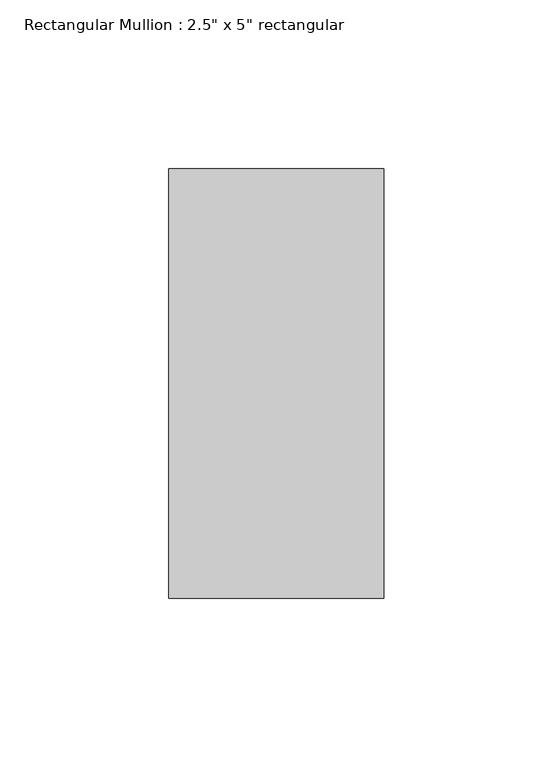
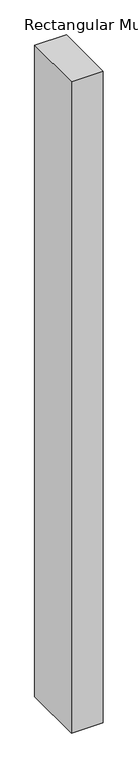
"""IFC4 building model written with IfcOpenShell, lengths in millimetres: member geometry."""

from ifc_helpers import new_model, si_unit, frame, origin, place, context, project, spatial, polyline, outline, extrude, source, transform, mapped, element, save


def member_faf5b19b(model_context):
    return source(origin(), model_context, "Body", "SweptSolid", [
        extrude(outline(polyline([(31.75, 63.5), (31.75, -63.5), (-31.75, -63.5), (-31.75, 63.5), (31.75, 63.5)])), frame((0.0, 0.0, -1377.9500001), z_axis=(0.0, 0.0, 1.0), x_axis=(1.0, 0.0, 0.0)), (0.0, 0.0, 1.0), 1377.9500001),
    ])


if __name__ == "__main__":
    model = new_model("IFC4")
    model_context = context("Model", 3, world=origin())
    ifc_project = project(units=[si_unit("LENGTHUNIT", "METRE", prefix="MILLI")], contexts=[model_context])
    site = spatial("IfcSite", under=ifc_project)
    building = spatial("IfcBuilding", under=site)
    placement = place(None, origin())
    member_shape = member_faf5b19b(model_context)
    element("IfcMember", 1, ObjectType="Rectangular Mullion : 2.5\" x 5\" rectangular", at=placement, inside=building, context=model_context, shape_type="MappedRepresentation", body=[
        mapped(member_shape, transform((0.0, 0.0, 0.0), x_axis=(1.0, 0.0, 0.0), y_axis=(0.0, 1.0, 0.0), z_axis=(0.0, 0.0, 1.0))),
    ])
    save(model, "model.ifc")

# Revit data of these elements
# Type "Rectangular Mullion : 2.5\" x 5\" rectangular"
#   built-in parameter 1007304 = 0.416667 (stored number, unit not read)
#   built-in parameter 1007301 = 0.104167 (stored number, unit not read)
#   built-in parameter 1007300 = 0.104167 (stored number, unit not read)
# Element 1 (IfcMember, "Rectangular Mullion : 2.5\" x 5\" rectangular")
#   Materials on its faces: "WINDOW FRAMING"
# Materials
#   "WINDOW FRAMING": class "Generic", colour RGB 120 120 120, transparency 0, Cost = 0
